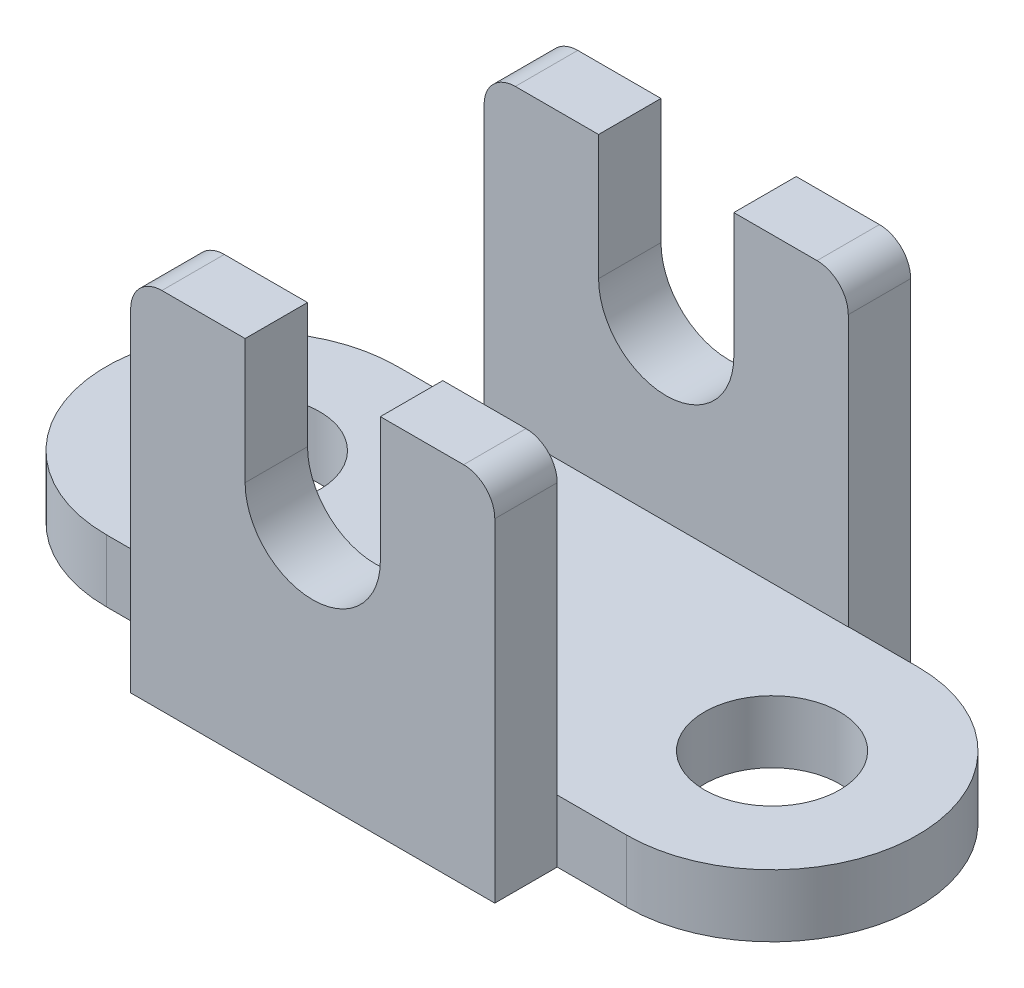
ISO-10303-21;
HEADER;
FILE_DESCRIPTION(('STEP AP214'),'2;1');
FILE_NAME('part.step','',(''),(''),'','','');
FILE_SCHEMA(('AUTOMOTIVE_DESIGN { 1 0 10303 214 1 1 1 1 }'));
ENDSEC;
DATA;
#1=APPLICATION_CONTEXT('core data for automotive mechanical design processes');
#2=APPLICATION_PROTOCOL_DEFINITION('international standard','automotive_design',2000,#1);
#3=PRODUCT_CONTEXT('',#1,'mechanical');
#4=PRODUCT('Part','Part','',(#3));
#5=PRODUCT_RELATED_PRODUCT_CATEGORY('part','',(#4));
#6=PRODUCT_DEFINITION_FORMATION('','',#4);
#7=PRODUCT_DEFINITION_CONTEXT('part definition',#1,'design');
#8=PRODUCT_DEFINITION('design','',#6,#7);
#9=PRODUCT_DEFINITION_SHAPE('','',#8);
#10=(LENGTH_UNIT() NAMED_UNIT(*) SI_UNIT(.MILLI.,.METRE.));
#11=(NAMED_UNIT(*) PLANE_ANGLE_UNIT() SI_UNIT($,.RADIAN.));
#12=(NAMED_UNIT(*) SI_UNIT($,.STERADIAN.) SOLID_ANGLE_UNIT());
#13=UNCERTAINTY_MEASURE_WITH_UNIT(LENGTH_MEASURE(1.E-05),#10,'distance_accuracy_value','');
#14=(GEOMETRIC_REPRESENTATION_CONTEXT(3) GLOBAL_UNCERTAINTY_ASSIGNED_CONTEXT((#13)) GLOBAL_UNIT_ASSIGNED_CONTEXT((#10,
#11,#12)) REPRESENTATION_CONTEXT('',''));
#15=CARTESIAN_POINT('',(0.,0.,0.));
#16=DIRECTION('',(0.,0.,1.));
#17=DIRECTION('',(1.,0.,0.));
#18=AXIS2_PLACEMENT_3D('',#15,#16,#17);
#19=CARTESIAN_POINT('',(-35.5583760815916,6.,33.9743802217869));
#20=DIRECTION('',(0.,0.,1.));
#21=DIRECTION('',(1.,0.,0.));
#22=AXIS2_PLACEMENT_3D('',#19,#20,#21);
#23=PLANE('',#22);
#24=DIRECTION('',(-1.,0.,0.));
#25=VECTOR('',#24,1.);
#26=CARTESIAN_POINT('',(-35.5583760815916,0.,33.9743802217869));
#27=LINE('',#26,#25);
#28=CARTESIAN_POINT('',(-27.2117962466488,0.,33.9743802217869));
#29=VERTEX_POINT('',#28);
#30=CARTESIAN_POINT('',(-35.5583760815916,0.,33.9743802217869));
#31=VERTEX_POINT('',#30);
#32=EDGE_CURVE('E281',#29,#31,#27,.T.);
#33=ORIENTED_EDGE('',*,*,#32,.F.);
#34=DIRECTION('',(0.,1.,0.));
#35=VECTOR('',#34,1.);
#36=CARTESIAN_POINT('',(-27.2117962466488,6.,33.9743802217869));
#37=LINE('',#36,#35);
#38=CARTESIAN_POINT('',(-27.2117962466488,6.,33.9743802217869));
#39=VERTEX_POINT('',#38);
#40=EDGE_CURVE('E11',#29,#39,#37,.T.);
#41=ORIENTED_EDGE('',*,*,#40,.T.);
#42=DIRECTION('',(-1.,0.,0.));
#43=VECTOR('',#42,1.);
#44=CARTESIAN_POINT('',(-35.5583760815916,6.,33.9743802217869));
#45=LINE('',#44,#43);
#46=CARTESIAN_POINT('',(-35.5583760815916,6.,33.9743802217869));
#47=VERTEX_POINT('',#46);
#48=EDGE_CURVE('E271',#39,#47,#45,.T.);
#49=ORIENTED_EDGE('',*,*,#48,.T.);
#50=DIRECTION('',(0.,-1.,0.));
#51=VECTOR('',#50,1.);
#52=CARTESIAN_POINT('',(-35.5583760815916,6.,33.9743802217869));
#53=LINE('',#52,#51);
#54=EDGE_CURVE('E290',#47,#31,#53,.T.);
#55=ORIENTED_EDGE('',*,*,#54,.T.);
#56=EDGE_LOOP('',(#33,#41,#49,#55));
#57=FACE_BOUND('',#56,.T.);
#58=ADVANCED_FACE('F39',(#57),#23,.T.);
#59=CARTESIAN_POINT('',(14.4416239184084,6.,33.9743802217869));
#60=VERTEX_POINT('',#59);
#61=CARTESIAN_POINT('',(7.7882037533512,6.,33.9743802217869));
#62=VERTEX_POINT('',#61);
#63=EDGE_CURVE('E275',#60,#62,#45,.T.);
#64=ORIENTED_EDGE('',*,*,#63,.T.);
#65=DIRECTION('',(0.,1.,0.));
#66=VECTOR('',#65,1.);
#67=CARTESIAN_POINT('',(7.7882037533512,0.,33.9743802217869));
#68=LINE('',#67,#66);
#69=CARTESIAN_POINT('',(7.7882037533512,0.,33.9743802217869));
#70=VERTEX_POINT('',#69);
#71=EDGE_CURVE('E392',#70,#62,#68,.T.);
#72=ORIENTED_EDGE('',*,*,#71,.F.);
#73=CARTESIAN_POINT('',(14.4416239184084,0.,33.9743802217869));
#74=VERTEX_POINT('',#73);
#75=EDGE_CURVE('E262',#74,#70,#27,.T.);
#76=ORIENTED_EDGE('',*,*,#75,.F.);
#77=DIRECTION('',(0.,-1.,0.));
#78=VECTOR('',#77,1.);
#79=CARTESIAN_POINT('',(14.4416239184084,6.,33.9743802217869));
#80=LINE('',#79,#78);
#81=EDGE_CURVE('E292',#60,#74,#80,.T.);
#82=ORIENTED_EDGE('',*,*,#81,.F.);
#83=EDGE_LOOP('',(#64,#72,#76,#82));
#84=FACE_BOUND('',#83,.T.);
#85=ADVANCED_FACE('F388',(#84),#23,.T.);
#86=CARTESIAN_POINT('',(-24.2117962466488,32.,6.));
#87=DIRECTION('',(0.,0.,1.));
#88=DIRECTION('',(1.,0.,0.));
#89=AXIS2_PLACEMENT_3D('',#86,#87,#88);
#90=PLANE('',#89);
#91=DIRECTION('',(0.,-1.,0.));
#92=VECTOR('',#91,1.);
#93=CARTESIAN_POINT('',(-27.2117962466488,0.,6.));
#94=LINE('',#93,#92);
#95=CARTESIAN_POINT('',(-27.2117962466488,32.,6.));
#96=VERTEX_POINT('',#95);
#97=CARTESIAN_POINT('',(-27.2117962466488,6.,6.));
#98=VERTEX_POINT('',#97);
#99=EDGE_CURVE('E301',#96,#98,#94,.T.);
#100=ORIENTED_EDGE('',*,*,#99,.T.);
#101=DIRECTION('',(1.,0.,0.));
#102=VECTOR('',#101,1.);
#103=CARTESIAN_POINT('',(-24.2117962466488,6.,6.));
#104=LINE('',#103,#102);
#105=CARTESIAN_POINT('',(7.7882037533512,6.,6.));
#106=VERTEX_POINT('',#105);
#107=EDGE_CURVE('E371',#98,#106,#104,.T.);
#108=ORIENTED_EDGE('',*,*,#107,.T.);
#109=DIRECTION('',(0.,1.,0.));
#110=VECTOR('',#109,1.);
#111=CARTESIAN_POINT('',(7.7882037533512,0.,6.));
#112=LINE('',#111,#110);
#113=CARTESIAN_POINT('',(7.7882037533512,32.,6.));
#114=VERTEX_POINT('',#113);
#115=EDGE_CURVE('E308',#106,#114,#112,.T.);
#116=ORIENTED_EDGE('',*,*,#115,.T.);
#117=CARTESIAN_POINT('',(4.7882037533512,32.,6.));
#118=DIRECTION('',(0.,0.,1.));
#119=DIRECTION('',(1.,0.,0.));
#120=AXIS2_PLACEMENT_3D('',#117,#118,#119);
#121=CIRCLE('',#120,3.);
#122=CARTESIAN_POINT('',(4.78820375335118,35.,6.));
#123=VERTEX_POINT('',#122);
#124=EDGE_CURVE('E310',#114,#123,#121,.T.);
#125=ORIENTED_EDGE('',*,*,#124,.T.);
#126=DIRECTION('',(-1.,0.,0.));
#127=VECTOR('',#126,1.);
#128=CARTESIAN_POINT('',(-3.2117962466488,35.,6.));
#129=LINE('',#128,#127);
#130=CARTESIAN_POINT('',(-3.2117962466488,35.,6.));
#131=VERTEX_POINT('',#130);
#132=EDGE_CURVE('E313',#123,#131,#129,.T.);
#133=ORIENTED_EDGE('',*,*,#132,.T.);
#134=DIRECTION('',(0.,-1.,0.));
#135=VECTOR('',#134,1.);
#136=CARTESIAN_POINT('',(-3.2117962466488,23.,6.));
#137=LINE('',#136,#135);
#138=CARTESIAN_POINT('',(-3.2117962466488,23.,6.));
#139=VERTEX_POINT('',#138);
#140=EDGE_CURVE('E311',#131,#139,#137,.T.);
#141=ORIENTED_EDGE('',*,*,#140,.T.);
#142=CARTESIAN_POINT('',(-9.7117962466488,23.,6.));
#143=DIRECTION('',(0.,0.,-1.));
#144=DIRECTION('',(1.,0.,0.));
#145=AXIS2_PLACEMENT_3D('',#142,#143,#144);
#146=CIRCLE('',#145,6.5);
#147=CARTESIAN_POINT('',(-16.2117962466488,23.,6.));
#148=VERTEX_POINT('',#147);
#149=EDGE_CURVE('E312',#139,#148,#146,.T.);
#150=ORIENTED_EDGE('',*,*,#149,.T.);
#151=DIRECTION('',(0.,1.,0.));
#152=VECTOR('',#151,1.);
#153=CARTESIAN_POINT('',(-16.2117962466488,35.,6.));
#154=LINE('',#153,#152);
#155=CARTESIAN_POINT('',(-16.2117962466488,35.,6.));
#156=VERTEX_POINT('',#155);
#157=EDGE_CURVE('E320',#148,#156,#154,.T.);
#158=ORIENTED_EDGE('',*,*,#157,.T.);
#159=DIRECTION('',(-1.,0.,0.));
#160=VECTOR('',#159,1.);
#161=CARTESIAN_POINT('',(-24.2117962466488,35.,6.));
#162=LINE('',#161,#160);
#163=CARTESIAN_POINT('',(-24.2117962466488,35.,6.));
#164=VERTEX_POINT('',#163);
#165=EDGE_CURVE('E317',#156,#164,#162,.T.);
#166=ORIENTED_EDGE('',*,*,#165,.T.);
#167=CARTESIAN_POINT('',(-24.2117962466488,32.,6.));
#168=DIRECTION('',(0.,0.,1.));
#169=DIRECTION('',(1.,0.,0.));
#170=AXIS2_PLACEMENT_3D('',#167,#168,#169);
#171=CIRCLE('',#170,3.);
#172=EDGE_CURVE('E321',#164,#96,#171,.T.);
#173=ORIENTED_EDGE('',*,*,#172,.T.);
#174=EDGE_LOOP('',(#100,#108,#116,#125,#133,#141,#150,#158,#166,#173));
#175=FACE_BOUND('',#174,.T.);
#176=ADVANCED_FACE('F533',(#175),#90,.T.);
#177=CARTESIAN_POINT('',(-27.2117962466488,0.,6.));
#178=DIRECTION('',(1.,0.,0.));
#179=DIRECTION('',(0.,0.,-1.));
#180=AXIS2_PLACEMENT_3D('',#177,#178,#179);
#181=PLANE('',#180);
#182=DIRECTION('',(0.,0.,-1.));
#183=VECTOR('',#182,1.);
#184=CARTESIAN_POINT('',(-27.2117962466488,0.,6.));
#185=LINE('',#184,#183);
#186=CARTESIAN_POINT('',(-27.2117962466488,0.,5.97438022178687));
#187=VERTEX_POINT('',#186);
#188=CARTESIAN_POINT('',(-27.2117962466488,0.,0.));
#189=VERTEX_POINT('',#188);
#190=EDGE_CURVE('E369',#187,#189,#185,.T.);
#191=ORIENTED_EDGE('',*,*,#190,.F.);
#192=DIRECTION('',(0.,1.,0.));
#193=VECTOR('',#192,1.);
#194=CARTESIAN_POINT('',(-27.2117962466488,0.,5.97438022178687));
#195=LINE('',#194,#193);
#196=CARTESIAN_POINT('',(-27.2117962466488,6.,5.97438022178687));
#197=VERTEX_POINT('',#196);
#198=EDGE_CURVE('E65',#187,#197,#195,.T.);
#199=ORIENTED_EDGE('',*,*,#198,.T.);
#200=DIRECTION('',(0.,0.,-1.));
#201=VECTOR('',#200,1.);
#202=CARTESIAN_POINT('',(-27.2117962466488,6.,6.));
#203=LINE('',#202,#201);
#204=EDGE_CURVE('E299',#98,#197,#203,.T.);
#205=ORIENTED_EDGE('',*,*,#204,.F.);
#206=ORIENTED_EDGE('',*,*,#99,.F.);
#207=DIRECTION('',(0.,0.,-1.));
#208=VECTOR('',#207,1.);
#209=CARTESIAN_POINT('',(-27.2117962466488,32.,6.));
#210=LINE('',#209,#208);
#211=CARTESIAN_POINT('',(-27.2117962466488,32.,0.));
#212=VERTEX_POINT('',#211);
#213=EDGE_CURVE('E323',#96,#212,#210,.T.);
#214=ORIENTED_EDGE('',*,*,#213,.T.);
#215=DIRECTION('',(0.,-1.,0.));
#216=VECTOR('',#215,1.);
#217=CARTESIAN_POINT('',(-27.2117962466488,0.,0.));
#218=LINE('',#217,#216);
#219=EDGE_CURVE('E305',#212,#189,#218,.T.);
#220=ORIENTED_EDGE('',*,*,#219,.T.);
#221=EDGE_LOOP('',(#191,#199,#205,#206,#214,#220));
#222=FACE_BOUND('',#221,.T.);
#223=ADVANCED_FACE('F41',(#222),#181,.F.);
#224=CARTESIAN_POINT('',(-27.2117962466488,0.,6.));
#225=DIRECTION('',(0.,1.,0.));
#226=DIRECTION('',(0.,0.,1.));
#227=AXIS2_PLACEMENT_3D('',#224,#225,#226);
#228=PLANE('',#227);
#229=CARTESIAN_POINT('',(-35.5583760815916,0.,19.9743802217869));
#230=DIRECTION('',(0.,1.,0.));
#231=DIRECTION('',(0.,0.,1.));
#232=AXIS2_PLACEMENT_3D('',#229,#230,#231);
#233=CIRCLE('',#232,6.5);
#234=CARTESIAN_POINT('',(-35.5583760815916,0.,26.4743802217869));
#235=VERTEX_POINT('',#234);
#236=EDGE_CURVE('E253',#235,#235,#233,.T.);
#237=ORIENTED_EDGE('',*,*,#236,.T.);
#238=EDGE_LOOP('',(#237));
#239=FACE_BOUND('',#238,.T.);
#240=CARTESIAN_POINT('',(14.4416239184084,0.,19.9743802217869));
#241=DIRECTION('',(0.,1.,0.));
#242=DIRECTION('',(0.,0.,1.));
#243=AXIS2_PLACEMENT_3D('',#240,#241,#242);
#244=CIRCLE('',#243,6.5);
#245=CARTESIAN_POINT('',(14.4416239184084,0.,26.4743802217869));
#246=VERTEX_POINT('',#245);
#247=EDGE_CURVE('E245',#246,#246,#244,.T.);
#248=ORIENTED_EDGE('',*,*,#247,.T.);
#249=EDGE_LOOP('',(#248));
#250=FACE_BOUND('',#249,.T.);
#251=DIRECTION('',(1.,0.,0.));
#252=VECTOR('',#251,1.);
#253=CARTESIAN_POINT('',(-35.5583760815916,0.,5.97438022178687));
#254=LINE('',#253,#252);
#255=CARTESIAN_POINT('',(-35.5583760815916,0.,5.97438022178687));
#256=VERTEX_POINT('',#255);
#257=EDGE_CURVE('E278',#256,#187,#254,.T.);
#258=ORIENTED_EDGE('',*,*,#257,.T.);
#259=ORIENTED_EDGE('',*,*,#190,.T.);
#260=DIRECTION('',(1.,0.,0.));
#261=VECTOR('',#260,1.);
#262=CARTESIAN_POINT('',(-27.2117962466488,0.,0.));
#263=LINE('',#262,#261);
#264=CARTESIAN_POINT('',(7.7882037533512,0.,0.));
#265=VERTEX_POINT('',#264);
#266=EDGE_CURVE('E326',#189,#265,#263,.T.);
#267=ORIENTED_EDGE('',*,*,#266,.T.);
#268=DIRECTION('',(0.,0.,-1.));
#269=VECTOR('',#268,1.);
#270=CARTESIAN_POINT('',(7.7882037533512,0.,6.));
#271=LINE('',#270,#269);
#272=CARTESIAN_POINT('',(7.7882037533512,0.,5.97438022178687));
#273=VERTEX_POINT('',#272);
#274=EDGE_CURVE('E370',#273,#265,#271,.T.);
#275=ORIENTED_EDGE('',*,*,#274,.F.);
#276=CARTESIAN_POINT('',(14.4416239184084,0.,5.97438022178687));
#277=VERTEX_POINT('',#276);
#278=EDGE_CURVE('E276',#273,#277,#254,.T.);
#279=ORIENTED_EDGE('',*,*,#278,.T.);
#280=CARTESIAN_POINT('',(14.4416239184084,0.,19.9743802217869));
#281=DIRECTION('',(0.,-1.,0.));
#282=DIRECTION('',(0.,0.,-1.));
#283=AXIS2_PLACEMENT_3D('',#280,#281,#282);
#284=CIRCLE('',#283,14.);
#285=EDGE_CURVE('E285',#277,#74,#284,.T.);
#286=ORIENTED_EDGE('',*,*,#285,.T.);
#287=ORIENTED_EDGE('',*,*,#75,.T.);
#288=DIRECTION('',(0.,0.,-1.));
#289=VECTOR('',#288,1.);
#290=CARTESIAN_POINT('',(7.7882037533512,0.,39.9743802217869));
#291=LINE('',#290,#289);
#292=CARTESIAN_POINT('',(7.7882037533512,0.,39.9743802217869));
#293=VERTEX_POINT('',#292);
#294=EDGE_CURVE('E53',#293,#70,#291,.T.);
#295=ORIENTED_EDGE('',*,*,#294,.F.);
#296=DIRECTION('',(1.,0.,0.));
#297=VECTOR('',#296,1.);
#298=CARTESIAN_POINT('',(-27.2117962466488,0.,39.9743802217869));
#299=LINE('',#298,#297);
#300=CARTESIAN_POINT('',(-27.2117962466488,0.,39.9743802217869));
#301=VERTEX_POINT('',#300);
#302=EDGE_CURVE('E218',#301,#293,#299,.T.);
#303=ORIENTED_EDGE('',*,*,#302,.F.);
#304=DIRECTION('',(0.,0.,-1.));
#305=VECTOR('',#304,1.);
#306=CARTESIAN_POINT('',(-27.2117962466488,0.,39.9743802217869));
#307=LINE('',#306,#305);
#308=EDGE_CURVE('E221',#301,#29,#307,.T.);
#309=ORIENTED_EDGE('',*,*,#308,.T.);
#310=ORIENTED_EDGE('',*,*,#32,.T.);
#311=CARTESIAN_POINT('',(-35.5583760815916,0.,19.9743802217869));
#312=DIRECTION('',(0.,-1.,0.));
#313=DIRECTION('',(0.,0.,-1.));
#314=AXIS2_PLACEMENT_3D('',#311,#312,#313);
#315=CIRCLE('',#314,14.);
#316=EDGE_CURVE('E255',#31,#256,#315,.T.);
#317=ORIENTED_EDGE('',*,*,#316,.T.);
#318=EDGE_LOOP('',(#258,#259,#267,#275,#279,#286,#287,#295,#303,#309,#310,#317));
#319=FACE_BOUND('',#318,.T.);
#320=ADVANCED_FACE('F225',(#239,#250,#319),#228,.F.);
#321=CARTESIAN_POINT('',(7.7882037533512,0.,6.));
#322=DIRECTION('',(-1.,0.,0.));
#323=DIRECTION('',(0.,-1.,0.));
#324=AXIS2_PLACEMENT_3D('',#321,#322,#323);
#325=PLANE('',#324);
#326=DIRECTION('',(0.,0.,1.));
#327=VECTOR('',#326,1.);
#328=CARTESIAN_POINT('',(7.7882037533512,6.,6.));
#329=LINE('',#328,#327);
#330=CARTESIAN_POINT('',(7.7882037533512,6.,5.97438022178687));
#331=VERTEX_POINT('',#330);
#332=EDGE_CURVE('E289',#331,#106,#329,.T.);
#333=ORIENTED_EDGE('',*,*,#332,.F.);
#334=DIRECTION('',(0.,-1.,0.));
#335=VECTOR('',#334,1.);
#336=CARTESIAN_POINT('',(7.7882037533512,0.,5.97438022178687));
#337=LINE('',#336,#335);
#338=EDGE_CURVE('E50',#331,#273,#337,.T.);
#339=ORIENTED_EDGE('',*,*,#338,.T.);
#340=ORIENTED_EDGE('',*,*,#274,.T.);
#341=DIRECTION('',(0.,1.,0.));
#342=VECTOR('',#341,1.);
#343=CARTESIAN_POINT('',(7.7882037533512,0.,0.));
#344=LINE('',#343,#342);
#345=CARTESIAN_POINT('',(7.7882037533512,32.,0.));
#346=VERTEX_POINT('',#345);
#347=EDGE_CURVE('E328',#265,#346,#344,.T.);
#348=ORIENTED_EDGE('',*,*,#347,.T.);
#349=DIRECTION('',(0.,0.,-1.));
#350=VECTOR('',#349,1.);
#351=CARTESIAN_POINT('',(7.7882037533512,32.,6.));
#352=LINE('',#351,#350);
#353=EDGE_CURVE('E365',#114,#346,#352,.T.);
#354=ORIENTED_EDGE('',*,*,#353,.F.);
#355=ORIENTED_EDGE('',*,*,#115,.F.);
#356=EDGE_LOOP('',(#333,#339,#340,#348,#354,#355));
#357=FACE_BOUND('',#356,.T.);
#358=ADVANCED_FACE('F374',(#357),#325,.F.);
#359=CARTESIAN_POINT('',(4.7882037533512,32.,6.));
#360=DIRECTION('',(0.,0.,-1.));
#361=DIRECTION('',(-1.,0.,0.));
#362=AXIS2_PLACEMENT_3D('',#359,#360,#361);
#363=CYLINDRICAL_SURFACE('',#362,3.);
#364=CARTESIAN_POINT('',(4.7882037533512,32.,0.));
#365=DIRECTION('',(0.,0.,1.));
#366=DIRECTION('',(1.,0.,0.));
#367=AXIS2_PLACEMENT_3D('',#364,#365,#366);
#368=CIRCLE('',#367,3.);
#369=CARTESIAN_POINT('',(4.78820375335118,35.,0.));
#370=VERTEX_POINT('',#369);
#371=EDGE_CURVE('E332',#346,#370,#368,.T.);
#372=ORIENTED_EDGE('',*,*,#371,.T.);
#373=DIRECTION('',(0.,0.,-1.));
#374=VECTOR('',#373,1.);
#375=CARTESIAN_POINT('',(4.78820375335118,35.,6.));
#376=LINE('',#375,#374);
#377=EDGE_CURVE('E363',#123,#370,#376,.T.);
#378=ORIENTED_EDGE('',*,*,#377,.F.);
#379=ORIENTED_EDGE('',*,*,#124,.F.);
#380=ORIENTED_EDGE('',*,*,#353,.T.);
#381=EDGE_LOOP('',(#372,#378,#379,#380));
#382=FACE_BOUND('',#381,.T.);
#383=ADVANCED_FACE('F526',(#382),#363,.T.);
#384=CARTESIAN_POINT('',(-3.2117962466488,35.,6.));
#385=DIRECTION('',(0.,-1.,0.));
#386=DIRECTION('',(0.,0.,-1.));
#387=AXIS2_PLACEMENT_3D('',#384,#385,#386);
#388=PLANE('',#387);
#389=DIRECTION('',(-1.,0.,0.));
#390=VECTOR('',#389,1.);
#391=CARTESIAN_POINT('',(-3.2117962466488,35.,0.));
#392=LINE('',#391,#390);
#393=CARTESIAN_POINT('',(-3.2117962466488,35.,0.));
#394=VERTEX_POINT('',#393);
#395=EDGE_CURVE('E334',#370,#394,#392,.T.);
#396=ORIENTED_EDGE('',*,*,#395,.T.);
#397=DIRECTION('',(0.,0.,-1.));
#398=VECTOR('',#397,1.);
#399=CARTESIAN_POINT('',(-3.2117962466488,35.,6.));
#400=LINE('',#399,#398);
#401=EDGE_CURVE('E356',#131,#394,#400,.T.);
#402=ORIENTED_EDGE('',*,*,#401,.F.);
#403=ORIENTED_EDGE('',*,*,#132,.F.);
#404=ORIENTED_EDGE('',*,*,#377,.T.);
#405=EDGE_LOOP('',(#396,#402,#403,#404));
#406=FACE_BOUND('',#405,.T.);
#407=ADVANCED_FACE('F522',(#406),#388,.F.);
#408=CARTESIAN_POINT('',(-3.2117962466488,23.,6.));
#409=DIRECTION('',(1.,0.,0.));
#410=DIRECTION('',(0.,1.,0.));
#411=AXIS2_PLACEMENT_3D('',#408,#409,#410);
#412=PLANE('',#411);
#413=DIRECTION('',(0.,-1.,0.));
#414=VECTOR('',#413,1.);
#415=CARTESIAN_POINT('',(-3.2117962466488,23.,0.));
#416=LINE('',#415,#414);
#417=CARTESIAN_POINT('',(-3.2117962466488,23.,0.));
#418=VERTEX_POINT('',#417);
#419=EDGE_CURVE('E333',#394,#418,#416,.T.);
#420=ORIENTED_EDGE('',*,*,#419,.T.);
#421=DIRECTION('',(0.,0.,-1.));
#422=VECTOR('',#421,1.);
#423=CARTESIAN_POINT('',(-3.2117962466488,23.,6.));
#424=LINE('',#423,#422);
#425=EDGE_CURVE('E351',#139,#418,#424,.T.);
#426=ORIENTED_EDGE('',*,*,#425,.F.);
#427=ORIENTED_EDGE('',*,*,#140,.F.);
#428=ORIENTED_EDGE('',*,*,#401,.T.);
#429=EDGE_LOOP('',(#420,#426,#427,#428));
#430=FACE_BOUND('',#429,.T.);
#431=ADVANCED_FACE('F519',(#430),#412,.F.);
#432=CARTESIAN_POINT('',(-9.7117962466488,23.,6.));
#433=DIRECTION('',(0.,0.,-1.));
#434=DIRECTION('',(-1.,0.,0.));
#435=AXIS2_PLACEMENT_3D('',#432,#433,#434);
#436=CYLINDRICAL_SURFACE('',#435,6.5);
#437=CARTESIAN_POINT('',(-9.7117962466488,23.,0.));
#438=DIRECTION('',(0.,0.,-1.));
#439=DIRECTION('',(1.,0.,0.));
#440=AXIS2_PLACEMENT_3D('',#437,#438,#439);
#441=CIRCLE('',#440,6.5);
#442=CARTESIAN_POINT('',(-16.2117962466488,23.,0.));
#443=VERTEX_POINT('',#442);
#444=EDGE_CURVE('E340',#418,#443,#441,.T.);
#445=ORIENTED_EDGE('',*,*,#444,.T.);
#446=DIRECTION('',(0.,0.,-1.));
#447=VECTOR('',#446,1.);
#448=CARTESIAN_POINT('',(-16.2117962466488,23.,6.));
#449=LINE('',#448,#447);
#450=EDGE_CURVE('E355',#148,#443,#449,.T.);
#451=ORIENTED_EDGE('',*,*,#450,.F.);
#452=ORIENTED_EDGE('',*,*,#149,.F.);
#453=ORIENTED_EDGE('',*,*,#425,.T.);
#454=EDGE_LOOP('',(#445,#451,#452,#453));
#455=FACE_BOUND('',#454,.T.);
#456=ADVANCED_FACE('F514',(#455),#436,.F.);
#457=CARTESIAN_POINT('',(-16.2117962466488,35.,6.));
#458=DIRECTION('',(-1.,0.,0.));
#459=DIRECTION('',(0.,-1.,0.));
#460=AXIS2_PLACEMENT_3D('',#457,#458,#459);
#461=PLANE('',#460);
#462=DIRECTION('',(0.,1.,0.));
#463=VECTOR('',#462,1.);
#464=CARTESIAN_POINT('',(-16.2117962466488,35.,0.));
#465=LINE('',#464,#463);
#466=CARTESIAN_POINT('',(-16.2117962466488,35.,0.));
#467=VERTEX_POINT('',#466);
#468=EDGE_CURVE('E339',#443,#467,#465,.T.);
#469=ORIENTED_EDGE('',*,*,#468,.T.);
#470=DIRECTION('',(0.,0.,-1.));
#471=VECTOR('',#470,1.);
#472=CARTESIAN_POINT('',(-16.2117962466488,35.,6.));
#473=LINE('',#472,#471);
#474=EDGE_CURVE('E349',#156,#467,#473,.T.);
#475=ORIENTED_EDGE('',*,*,#474,.F.);
#476=ORIENTED_EDGE('',*,*,#157,.F.);
#477=ORIENTED_EDGE('',*,*,#450,.T.);
#478=EDGE_LOOP('',(#469,#475,#476,#477));
#479=FACE_BOUND('',#478,.T.);
#480=ADVANCED_FACE('F509',(#479),#461,.F.);
#481=CARTESIAN_POINT('',(-24.2117962466488,35.,6.));
#482=DIRECTION('',(0.,-1.,0.));
#483=DIRECTION('',(0.,0.,-1.));
#484=AXIS2_PLACEMENT_3D('',#481,#482,#483);
#485=PLANE('',#484);
#486=DIRECTION('',(-1.,0.,0.));
#487=VECTOR('',#486,1.);
#488=CARTESIAN_POINT('',(-24.2117962466488,35.,0.));
#489=LINE('',#488,#487);
#490=CARTESIAN_POINT('',(-24.2117962466488,35.,0.));
#491=VERTEX_POINT('',#490);
#492=EDGE_CURVE('E343',#467,#491,#489,.T.);
#493=ORIENTED_EDGE('',*,*,#492,.T.);
#494=DIRECTION('',(0.,0.,-1.));
#495=VECTOR('',#494,1.);
#496=CARTESIAN_POINT('',(-24.2117962466488,35.,6.));
#497=LINE('',#496,#495);
#498=EDGE_CURVE('E347',#164,#491,#497,.T.);
#499=ORIENTED_EDGE('',*,*,#498,.F.);
#500=ORIENTED_EDGE('',*,*,#165,.F.);
#501=ORIENTED_EDGE('',*,*,#474,.T.);
#502=EDGE_LOOP('',(#493,#499,#500,#501));
#503=FACE_BOUND('',#502,.T.);
#504=ADVANCED_FACE('F501',(#503),#485,.F.);
#505=CARTESIAN_POINT('',(-24.2117962466488,32.,6.));
#506=DIRECTION('',(0.,0.,-1.));
#507=DIRECTION('',(-1.,0.,0.));
#508=AXIS2_PLACEMENT_3D('',#505,#506,#507);
#509=CYLINDRICAL_SURFACE('',#508,3.);
#510=CARTESIAN_POINT('',(-24.2117962466488,32.,0.));
#511=DIRECTION('',(0.,0.,1.));
#512=DIRECTION('',(1.,0.,0.));
#513=AXIS2_PLACEMENT_3D('',#510,#511,#512);
#514=CIRCLE('',#513,3.);
#515=EDGE_CURVE('E307',#491,#212,#514,.T.);
#516=ORIENTED_EDGE('',*,*,#515,.T.);
#517=ORIENTED_EDGE('',*,*,#213,.F.);
#518=ORIENTED_EDGE('',*,*,#172,.F.);
#519=ORIENTED_EDGE('',*,*,#498,.T.);
#520=EDGE_LOOP('',(#516,#517,#518,#519));
#521=FACE_BOUND('',#520,.T.);
#522=ADVANCED_FACE('F496',(#521),#509,.T.);
#523=CARTESIAN_POINT('',(-24.2117962466488,32.,0.));
#524=DIRECTION('',(0.,0.,1.));
#525=DIRECTION('',(1.,0.,0.));
#526=AXIS2_PLACEMENT_3D('',#523,#524,#525);
#527=PLANE('',#526);
#528=ORIENTED_EDGE('',*,*,#219,.F.);
#529=ORIENTED_EDGE('',*,*,#515,.F.);
#530=ORIENTED_EDGE('',*,*,#492,.F.);
#531=ORIENTED_EDGE('',*,*,#468,.F.);
#532=ORIENTED_EDGE('',*,*,#444,.F.);
#533=ORIENTED_EDGE('',*,*,#419,.F.);
#534=ORIENTED_EDGE('',*,*,#395,.F.);
#535=ORIENTED_EDGE('',*,*,#371,.F.);
#536=ORIENTED_EDGE('',*,*,#347,.F.);
#537=ORIENTED_EDGE('',*,*,#266,.F.);
#538=EDGE_LOOP('',(#528,#529,#530,#531,#532,#533,#534,#535,#536,#537));
#539=FACE_BOUND('',#538,.T.);
#540=ADVANCED_FACE('F495',(#539),#527,.F.);
#541=CARTESIAN_POINT('',(-35.5583760815916,6.,5.97438022178687));
#542=DIRECTION('',(0.,0.,-1.));
#543=DIRECTION('',(-1.,0.,0.));
#544=AXIS2_PLACEMENT_3D('',#541,#542,#543);
#545=PLANE('',#544);
#546=ORIENTED_EDGE('',*,*,#198,.F.);
#547=ORIENTED_EDGE('',*,*,#257,.F.);
#548=DIRECTION('',(0.,-1.,0.));
#549=VECTOR('',#548,1.);
#550=CARTESIAN_POINT('',(-35.5583760815916,6.,5.97438022178687));
#551=LINE('',#550,#549);
#552=CARTESIAN_POINT('',(-35.5583760815916,6.,5.97438022178687));
#553=VERTEX_POINT('',#552);
#554=EDGE_CURVE('E274',#553,#256,#551,.T.);
#555=ORIENTED_EDGE('',*,*,#554,.F.);
#556=DIRECTION('',(1.,0.,0.));
#557=VECTOR('',#556,1.);
#558=CARTESIAN_POINT('',(-35.5583760815916,6.,5.97438022178687));
#559=LINE('',#558,#557);
#560=EDGE_CURVE('E264',#553,#197,#559,.T.);
#561=ORIENTED_EDGE('',*,*,#560,.T.);
#562=EDGE_LOOP('',(#546,#547,#555,#561));
#563=FACE_BOUND('',#562,.T.);
#564=ADVANCED_FACE('F488',(#563),#545,.T.);
#565=ORIENTED_EDGE('',*,*,#338,.F.);
#566=CARTESIAN_POINT('',(14.4416239184084,6.,5.97438022178687));
#567=VERTEX_POINT('',#566);
#568=EDGE_CURVE('E263',#331,#567,#559,.T.);
#569=ORIENTED_EDGE('',*,*,#568,.T.);
#570=DIRECTION('',(0.,-1.,0.));
#571=VECTOR('',#570,1.);
#572=CARTESIAN_POINT('',(14.4416239184084,6.,5.97438022178687));
#573=LINE('',#572,#571);
#574=EDGE_CURVE('E291',#567,#277,#573,.T.);
#575=ORIENTED_EDGE('',*,*,#574,.T.);
#576=ORIENTED_EDGE('',*,*,#278,.F.);
#577=EDGE_LOOP('',(#565,#569,#575,#576));
#578=FACE_BOUND('',#577,.T.);
#579=ADVANCED_FACE('F385',(#578),#545,.T.);
#580=CARTESIAN_POINT('',(-35.5583760815916,6.,19.9743802217869));
#581=DIRECTION('',(0.,-1.,0.));
#582=DIRECTION('',(0.,0.,-1.));
#583=AXIS2_PLACEMENT_3D('',#580,#581,#582);
#584=PLANE('',#583);
#585=CARTESIAN_POINT('',(-35.5583760815916,6.,19.9743802217869));
#586=DIRECTION('',(0.,1.,0.));
#587=DIRECTION('',(0.,0.,1.));
#588=AXIS2_PLACEMENT_3D('',#585,#586,#587);
#589=CIRCLE('',#588,6.5);
#590=CARTESIAN_POINT('',(-35.5583760815916,6.,26.4743802217869));
#591=VERTEX_POINT('',#590);
#592=EDGE_CURVE('E254',#591,#591,#589,.T.);
#593=ORIENTED_EDGE('',*,*,#592,.F.);
#594=EDGE_LOOP('',(#593));
#595=FACE_BOUND('',#594,.T.);
#596=CARTESIAN_POINT('',(14.4416239184084,6.,19.9743802217869));
#597=DIRECTION('',(0.,1.,0.));
#598=DIRECTION('',(0.,0.,1.));
#599=AXIS2_PLACEMENT_3D('',#596,#597,#598);
#600=CIRCLE('',#599,6.5);
#601=CARTESIAN_POINT('',(14.4416239184084,6.,26.4743802217869));
#602=VERTEX_POINT('',#601);
#603=EDGE_CURVE('E241',#602,#602,#600,.T.);
#604=ORIENTED_EDGE('',*,*,#603,.F.);
#605=EDGE_LOOP('',(#604));
#606=FACE_BOUND('',#605,.T.);
#607=ORIENTED_EDGE('',*,*,#107,.F.);
#608=ORIENTED_EDGE('',*,*,#204,.T.);
#609=ORIENTED_EDGE('',*,*,#560,.F.);
#610=CARTESIAN_POINT('',(-35.5583760815916,6.,19.9743802217869));
#611=DIRECTION('',(0.,-1.,0.));
#612=DIRECTION('',(0.,0.,-1.));
#613=AXIS2_PLACEMENT_3D('',#610,#611,#612);
#614=CIRCLE('',#613,14.);
#615=EDGE_CURVE('E257',#47,#553,#614,.T.);
#616=ORIENTED_EDGE('',*,*,#615,.F.);
#617=ORIENTED_EDGE('',*,*,#48,.F.);
#618=EDGE_CURVE('E277',#62,#39,#45,.T.);
#619=ORIENTED_EDGE('',*,*,#618,.F.);
#620=ORIENTED_EDGE('',*,*,#63,.F.);
#621=CARTESIAN_POINT('',(14.4416239184084,6.,19.9743802217869));
#622=DIRECTION('',(0.,-1.,0.));
#623=DIRECTION('',(0.,0.,-1.));
#624=AXIS2_PLACEMENT_3D('',#621,#622,#623);
#625=CIRCLE('',#624,14.);
#626=EDGE_CURVE('E268',#567,#60,#625,.T.);
#627=ORIENTED_EDGE('',*,*,#626,.F.);
#628=ORIENTED_EDGE('',*,*,#568,.F.);
#629=ORIENTED_EDGE('',*,*,#332,.T.);
#630=EDGE_LOOP('',(#607,#608,#609,#616,#617,#619,#620,#627,#628,#629));
#631=FACE_BOUND('',#630,.T.);
#632=ADVANCED_FACE('F486',(#595,#606,#631),#584,.F.);
#633=CARTESIAN_POINT('',(-35.5583760815916,6.,19.9743802217869));
#634=DIRECTION('',(0.,-1.,0.));
#635=DIRECTION('',(0.,0.,-1.));
#636=AXIS2_PLACEMENT_3D('',#633,#634,#635);
#637=CYLINDRICAL_SURFACE('',#636,14.);
#638=ORIENTED_EDGE('',*,*,#316,.F.);
#639=ORIENTED_EDGE('',*,*,#54,.F.);
#640=ORIENTED_EDGE('',*,*,#615,.T.);
#641=ORIENTED_EDGE('',*,*,#554,.T.);
#642=EDGE_LOOP('',(#638,#639,#640,#641));
#643=FACE_BOUND('',#642,.T.);
#644=ADVANCED_FACE('F483',(#643),#637,.T.);
#645=CARTESIAN_POINT('',(14.4416239184084,6.,19.9743802217869));
#646=DIRECTION('',(0.,-1.,0.));
#647=DIRECTION('',(0.,0.,-1.));
#648=AXIS2_PLACEMENT_3D('',#645,#646,#647);
#649=CYLINDRICAL_SURFACE('',#648,14.);
#650=ORIENTED_EDGE('',*,*,#285,.F.);
#651=ORIENTED_EDGE('',*,*,#574,.F.);
#652=ORIENTED_EDGE('',*,*,#626,.T.);
#653=ORIENTED_EDGE('',*,*,#81,.T.);
#654=EDGE_LOOP('',(#650,#651,#652,#653));
#655=FACE_BOUND('',#654,.T.);
#656=ADVANCED_FACE('F390',(#655),#649,.T.);
#657=CARTESIAN_POINT('',(14.4416239184084,0.,19.9743802217869));
#658=DIRECTION('',(0.,1.,0.));
#659=DIRECTION('',(0.,0.,1.));
#660=AXIS2_PLACEMENT_3D('',#657,#658,#659);
#661=CYLINDRICAL_SURFACE('',#660,6.5);
#662=ORIENTED_EDGE('',*,*,#247,.F.);
#663=EDGE_LOOP('',(#662));
#664=FACE_BOUND('',#663,.T.);
#665=ORIENTED_EDGE('',*,*,#603,.T.);
#666=EDGE_LOOP('',(#665));
#667=FACE_BOUND('',#666,.T.);
#668=ADVANCED_FACE('F552',(#664,#667),#661,.F.);
#669=CARTESIAN_POINT('',(-35.5583760815916,0.,19.9743802217869));
#670=DIRECTION('',(0.,1.,0.));
#671=DIRECTION('',(0.,0.,1.));
#672=AXIS2_PLACEMENT_3D('',#669,#670,#671);
#673=CYLINDRICAL_SURFACE('',#672,6.5);
#674=ORIENTED_EDGE('',*,*,#236,.F.);
#675=EDGE_LOOP('',(#674));
#676=FACE_BOUND('',#675,.T.);
#677=ORIENTED_EDGE('',*,*,#592,.T.);
#678=EDGE_LOOP('',(#677));
#679=FACE_BOUND('',#678,.T.);
#680=ADVANCED_FACE('F566',(#676,#679),#673,.F.);
#681=CARTESIAN_POINT('',(4.7882037533512,32.,33.9743802217869));
#682=DIRECTION('',(0.,0.,1.));
#683=DIRECTION('',(1.,0.,0.));
#684=AXIS2_PLACEMENT_3D('',#681,#682,#683);
#685=PLANE('',#684);
#686=CARTESIAN_POINT('',(7.7882037533512,32.,33.9743802217869));
#687=VERTEX_POINT('',#686);
#688=EDGE_CURVE('E391',#62,#687,#68,.T.);
#689=ORIENTED_EDGE('',*,*,#688,.F.);
#690=ORIENTED_EDGE('',*,*,#618,.T.);
#691=DIRECTION('',(0.,-1.,0.));
#692=VECTOR('',#691,1.);
#693=CARTESIAN_POINT('',(-27.2117962466488,32.,33.9743802217869));
#694=LINE('',#693,#692);
#695=CARTESIAN_POINT('',(-27.2117962466488,32.,33.9743802217869));
#696=VERTEX_POINT('',#695);
#697=EDGE_CURVE('E397',#696,#39,#694,.T.);
#698=ORIENTED_EDGE('',*,*,#697,.F.);
#699=CARTESIAN_POINT('',(-24.2117962466488,32.,33.9743802217869));
#700=DIRECTION('',(0.,0.,1.));
#701=DIRECTION('',(1.,0.,0.));
#702=AXIS2_PLACEMENT_3D('',#699,#700,#701);
#703=CIRCLE('',#702,3.);
#704=CARTESIAN_POINT('',(-24.2117962466488,35.,33.9743802217869));
#705=VERTEX_POINT('',#704);
#706=EDGE_CURVE('E236',#705,#696,#703,.T.);
#707=ORIENTED_EDGE('',*,*,#706,.F.);
#708=DIRECTION('',(-1.,0.,0.));
#709=VECTOR('',#708,1.);
#710=CARTESIAN_POINT('',(-16.2117962466488,35.,33.9743802217869));
#711=LINE('',#710,#709);
#712=CARTESIAN_POINT('',(-16.2117962466488,35.,33.9743802217869));
#713=VERTEX_POINT('',#712);
#714=EDGE_CURVE('E406',#713,#705,#711,.T.);
#715=ORIENTED_EDGE('',*,*,#714,.F.);
#716=DIRECTION('',(0.,1.,0.));
#717=VECTOR('',#716,1.);
#718=CARTESIAN_POINT('',(-16.2117962466488,35.,33.9743802217869));
#719=LINE('',#718,#717);
#720=CARTESIAN_POINT('',(-16.2117962466488,23.,33.9743802217869));
#721=VERTEX_POINT('',#720);
#722=EDGE_CURVE('E408',#721,#713,#719,.T.);
#723=ORIENTED_EDGE('',*,*,#722,.F.);
#724=CARTESIAN_POINT('',(-9.7117962466488,23.,33.9743802217869));
#725=DIRECTION('',(0.,0.,-1.));
#726=DIRECTION('',(1.,0.,0.));
#727=AXIS2_PLACEMENT_3D('',#724,#725,#726);
#728=CIRCLE('',#727,6.5);
#729=CARTESIAN_POINT('',(-3.2117962466488,23.,33.9743802217869));
#730=VERTEX_POINT('',#729);
#731=EDGE_CURVE('E407',#730,#721,#728,.T.);
#732=ORIENTED_EDGE('',*,*,#731,.F.);
#733=DIRECTION('',(0.,-1.,0.));
#734=VECTOR('',#733,1.);
#735=CARTESIAN_POINT('',(-3.2117962466488,23.,33.9743802217869));
#736=LINE('',#735,#734);
#737=CARTESIAN_POINT('',(-3.2117962466488,35.,33.9743802217869));
#738=VERTEX_POINT('',#737);
#739=EDGE_CURVE('E404',#738,#730,#736,.T.);
#740=ORIENTED_EDGE('',*,*,#739,.F.);
#741=DIRECTION('',(-1.,0.,0.));
#742=VECTOR('',#741,1.);
#743=CARTESIAN_POINT('',(4.78820375335118,35.,33.9743802217869));
#744=LINE('',#743,#742);
#745=CARTESIAN_POINT('',(4.78820375335118,35.,33.9743802217869));
#746=VERTEX_POINT('',#745);
#747=EDGE_CURVE('E400',#746,#738,#744,.T.);
#748=ORIENTED_EDGE('',*,*,#747,.F.);
#749=CARTESIAN_POINT('',(4.7882037533512,32.,33.9743802217869));
#750=DIRECTION('',(0.,0.,1.));
#751=DIRECTION('',(1.,0.,0.));
#752=AXIS2_PLACEMENT_3D('',#749,#750,#751);
#753=CIRCLE('',#752,3.);
#754=EDGE_CURVE('E394',#687,#746,#753,.T.);
#755=ORIENTED_EDGE('',*,*,#754,.F.);
#756=EDGE_LOOP('',(#689,#690,#698,#707,#715,#723,#732,#740,#748,#755));
#757=FACE_BOUND('',#756,.T.);
#758=ADVANCED_FACE('F445',(#757),#685,.F.);
#759=CARTESIAN_POINT('',(-27.2117962466488,32.,39.9743802217869));
#760=DIRECTION('',(1.,0.,0.));
#761=DIRECTION('',(0.,0.,-1.));
#762=AXIS2_PLACEMENT_3D('',#759,#760,#761);
#763=PLANE('',#762);
#764=ORIENTED_EDGE('',*,*,#697,.T.);
#765=ORIENTED_EDGE('',*,*,#40,.F.);
#766=ORIENTED_EDGE('',*,*,#308,.F.);
#767=DIRECTION('',(0.,-1.,0.));
#768=VECTOR('',#767,1.);
#769=CARTESIAN_POINT('',(-27.2117962466488,32.,39.9743802217869));
#770=LINE('',#769,#768);
#771=CARTESIAN_POINT('',(-27.2117962466488,32.,39.9743802217869));
#772=VERTEX_POINT('',#771);
#773=EDGE_CURVE('E229',#772,#301,#770,.T.);
#774=ORIENTED_EDGE('',*,*,#773,.F.);
#775=DIRECTION('',(0.,0.,-1.));
#776=VECTOR('',#775,1.);
#777=CARTESIAN_POINT('',(-27.2117962466488,32.,39.9743802217869));
#778=LINE('',#777,#776);
#779=EDGE_CURVE('E411',#772,#696,#778,.T.);
#780=ORIENTED_EDGE('',*,*,#779,.T.);
#781=EDGE_LOOP('',(#764,#765,#766,#774,#780));
#782=FACE_BOUND('',#781,.T.);
#783=ADVANCED_FACE('F242',(#782),#763,.F.);
#784=CARTESIAN_POINT('',(7.7882037533512,0.,39.9743802217869));
#785=DIRECTION('',(-1.,0.,0.));
#786=DIRECTION('',(0.,0.,1.));
#787=AXIS2_PLACEMENT_3D('',#784,#785,#786);
#788=PLANE('',#787);
#789=ORIENTED_EDGE('',*,*,#71,.T.);
#790=ORIENTED_EDGE('',*,*,#688,.T.);
#791=DIRECTION('',(0.,0.,-1.));
#792=VECTOR('',#791,1.);
#793=CARTESIAN_POINT('',(7.7882037533512,32.,39.9743802217869));
#794=LINE('',#793,#792);
#795=CARTESIAN_POINT('',(7.7882037533512,32.,39.9743802217869));
#796=VERTEX_POINT('',#795);
#797=EDGE_CURVE('E250',#796,#687,#794,.T.);
#798=ORIENTED_EDGE('',*,*,#797,.F.);
#799=DIRECTION('',(0.,1.,0.));
#800=VECTOR('',#799,1.);
#801=CARTESIAN_POINT('',(7.7882037533512,0.,39.9743802217869));
#802=LINE('',#801,#800);
#803=EDGE_CURVE('E228',#293,#796,#802,.T.);
#804=ORIENTED_EDGE('',*,*,#803,.F.);
#805=ORIENTED_EDGE('',*,*,#294,.T.);
#806=EDGE_LOOP('',(#789,#790,#798,#804,#805));
#807=FACE_BOUND('',#806,.T.);
#808=ADVANCED_FACE('F576',(#807),#788,.F.);
#809=CARTESIAN_POINT('',(4.7882037533512,32.,39.9743802217869));
#810=DIRECTION('',(0.,0.,-1.));
#811=DIRECTION('',(-1.,0.,0.));
#812=AXIS2_PLACEMENT_3D('',#809,#810,#811);
#813=CYLINDRICAL_SURFACE('',#812,3.);
#814=ORIENTED_EDGE('',*,*,#754,.T.);
#815=DIRECTION('',(0.,0.,-1.));
#816=VECTOR('',#815,1.);
#817=CARTESIAN_POINT('',(4.78820375335118,35.,39.9743802217869));
#818=LINE('',#817,#816);
#819=CARTESIAN_POINT('',(4.78820375335118,35.,39.9743802217869));
#820=VERTEX_POINT('',#819);
#821=EDGE_CURVE('E429',#820,#746,#818,.T.);
#822=ORIENTED_EDGE('',*,*,#821,.F.);
#823=CARTESIAN_POINT('',(4.7882037533512,32.,39.9743802217869));
#824=DIRECTION('',(0.,0.,1.));
#825=DIRECTION('',(1.,0.,0.));
#826=AXIS2_PLACEMENT_3D('',#823,#824,#825);
#827=CIRCLE('',#826,3.);
#828=EDGE_CURVE('E438',#796,#820,#827,.T.);
#829=ORIENTED_EDGE('',*,*,#828,.F.);
#830=ORIENTED_EDGE('',*,*,#797,.T.);
#831=EDGE_LOOP('',(#814,#822,#829,#830));
#832=FACE_BOUND('',#831,.T.);
#833=ADVANCED_FACE('F440',(#832),#813,.T.);
#834=CARTESIAN_POINT('',(4.78820375335118,35.,39.9743802217869));
#835=DIRECTION('',(0.,-1.,0.));
#836=DIRECTION('',(0.,0.,-1.));
#837=AXIS2_PLACEMENT_3D('',#834,#835,#836);
#838=PLANE('',#837);
#839=ORIENTED_EDGE('',*,*,#747,.T.);
#840=DIRECTION('',(0.,0.,-1.));
#841=VECTOR('',#840,1.);
#842=CARTESIAN_POINT('',(-3.2117962466488,35.,39.9743802217869));
#843=LINE('',#842,#841);
#844=CARTESIAN_POINT('',(-3.2117962466488,35.,39.9743802217869));
#845=VERTEX_POINT('',#844);
#846=EDGE_CURVE('E430',#845,#738,#843,.T.);
#847=ORIENTED_EDGE('',*,*,#846,.F.);
#848=DIRECTION('',(-1.,0.,0.));
#849=VECTOR('',#848,1.);
#850=CARTESIAN_POINT('',(4.78820375335118,35.,39.9743802217869));
#851=LINE('',#850,#849);
#852=EDGE_CURVE('E457',#820,#845,#851,.T.);
#853=ORIENTED_EDGE('',*,*,#852,.F.);
#854=ORIENTED_EDGE('',*,*,#821,.T.);
#855=EDGE_LOOP('',(#839,#847,#853,#854));
#856=FACE_BOUND('',#855,.T.);
#857=ADVANCED_FACE('F450',(#856),#838,.F.);
#858=CARTESIAN_POINT('',(-3.2117962466488,23.,39.9743802217869));
#859=DIRECTION('',(1.,0.,0.));
#860=DIRECTION('',(0.,1.,0.));
#861=AXIS2_PLACEMENT_3D('',#858,#859,#860);
#862=PLANE('',#861);
#863=ORIENTED_EDGE('',*,*,#739,.T.);
#864=DIRECTION('',(0.,0.,-1.));
#865=VECTOR('',#864,1.);
#866=CARTESIAN_POINT('',(-3.2117962466488,23.,39.9743802217869));
#867=LINE('',#866,#865);
#868=CARTESIAN_POINT('',(-3.2117962466488,23.,39.9743802217869));
#869=VERTEX_POINT('',#868);
#870=EDGE_CURVE('E424',#869,#730,#867,.T.);
#871=ORIENTED_EDGE('',*,*,#870,.F.);
#872=DIRECTION('',(0.,-1.,0.));
#873=VECTOR('',#872,1.);
#874=CARTESIAN_POINT('',(-3.2117962466488,23.,39.9743802217869));
#875=LINE('',#874,#873);
#876=EDGE_CURVE('E451',#845,#869,#875,.T.);
#877=ORIENTED_EDGE('',*,*,#876,.F.);
#878=ORIENTED_EDGE('',*,*,#846,.T.);
#879=EDGE_LOOP('',(#863,#871,#877,#878));
#880=FACE_BOUND('',#879,.T.);
#881=ADVANCED_FACE('F453',(#880),#862,.F.);
#882=CARTESIAN_POINT('',(-9.7117962466488,23.,39.9743802217869));
#883=DIRECTION('',(0.,0.,-1.));
#884=DIRECTION('',(-1.,0.,0.));
#885=AXIS2_PLACEMENT_3D('',#882,#883,#884);
#886=CYLINDRICAL_SURFACE('',#885,6.5);
#887=ORIENTED_EDGE('',*,*,#731,.T.);
#888=DIRECTION('',(0.,0.,-1.));
#889=VECTOR('',#888,1.);
#890=CARTESIAN_POINT('',(-16.2117962466488,23.,39.9743802217869));
#891=LINE('',#890,#889);
#892=CARTESIAN_POINT('',(-16.2117962466488,23.,39.9743802217869));
#893=VERTEX_POINT('',#892);
#894=EDGE_CURVE('E423',#893,#721,#891,.T.);
#895=ORIENTED_EDGE('',*,*,#894,.F.);
#896=CARTESIAN_POINT('',(-9.7117962466488,23.,39.9743802217869));
#897=DIRECTION('',(0.,0.,-1.));
#898=DIRECTION('',(1.,0.,0.));
#899=AXIS2_PLACEMENT_3D('',#896,#897,#898);
#900=CIRCLE('',#899,6.5);
#901=EDGE_CURVE('E454',#869,#893,#900,.T.);
#902=ORIENTED_EDGE('',*,*,#901,.F.);
#903=ORIENTED_EDGE('',*,*,#870,.T.);
#904=EDGE_LOOP('',(#887,#895,#902,#903));
#905=FACE_BOUND('',#904,.T.);
#906=ADVANCED_FACE('F590',(#905),#886,.F.);
#907=CARTESIAN_POINT('',(-16.2117962466488,35.,39.9743802217869));
#908=DIRECTION('',(-1.,0.,0.));
#909=DIRECTION('',(0.,-1.,0.));
#910=AXIS2_PLACEMENT_3D('',#907,#908,#909);
#911=PLANE('',#910);
#912=ORIENTED_EDGE('',*,*,#722,.T.);
#913=DIRECTION('',(0.,0.,-1.));
#914=VECTOR('',#913,1.);
#915=CARTESIAN_POINT('',(-16.2117962466488,35.,39.9743802217869));
#916=LINE('',#915,#914);
#917=CARTESIAN_POINT('',(-16.2117962466488,35.,39.9743802217869));
#918=VERTEX_POINT('',#917);
#919=EDGE_CURVE('E416',#918,#713,#916,.T.);
#920=ORIENTED_EDGE('',*,*,#919,.F.);
#921=DIRECTION('',(0.,1.,0.));
#922=VECTOR('',#921,1.);
#923=CARTESIAN_POINT('',(-16.2117962466488,35.,39.9743802217869));
#924=LINE('',#923,#922);
#925=EDGE_CURVE('E456',#893,#918,#924,.T.);
#926=ORIENTED_EDGE('',*,*,#925,.F.);
#927=ORIENTED_EDGE('',*,*,#894,.T.);
#928=EDGE_LOOP('',(#912,#920,#926,#927));
#929=FACE_BOUND('',#928,.T.);
#930=ADVANCED_FACE('F587',(#929),#911,.F.);
#931=CARTESIAN_POINT('',(-16.2117962466488,35.,39.9743802217869));
#932=DIRECTION('',(0.,-1.,0.));
#933=DIRECTION('',(0.,0.,-1.));
#934=AXIS2_PLACEMENT_3D('',#931,#932,#933);
#935=PLANE('',#934);
#936=ORIENTED_EDGE('',*,*,#714,.T.);
#937=DIRECTION('',(0.,0.,-1.));
#938=VECTOR('',#937,1.);
#939=CARTESIAN_POINT('',(-24.2117962466488,35.,39.9743802217869));
#940=LINE('',#939,#938);
#941=CARTESIAN_POINT('',(-24.2117962466488,35.,39.9743802217869));
#942=VERTEX_POINT('',#941);
#943=EDGE_CURVE('E414',#942,#705,#940,.T.);
#944=ORIENTED_EDGE('',*,*,#943,.F.);
#945=DIRECTION('',(-1.,0.,0.));
#946=VECTOR('',#945,1.);
#947=CARTESIAN_POINT('',(-16.2117962466488,35.,39.9743802217869));
#948=LINE('',#947,#946);
#949=EDGE_CURVE('E464',#918,#942,#948,.T.);
#950=ORIENTED_EDGE('',*,*,#949,.F.);
#951=ORIENTED_EDGE('',*,*,#919,.T.);
#952=EDGE_LOOP('',(#936,#944,#950,#951));
#953=FACE_BOUND('',#952,.T.);
#954=ADVANCED_FACE('F469',(#953),#935,.F.);
#955=CARTESIAN_POINT('',(-24.2117962466488,32.,39.9743802217869));
#956=DIRECTION('',(0.,0.,-1.));
#957=DIRECTION('',(-1.,0.,0.));
#958=AXIS2_PLACEMENT_3D('',#955,#956,#957);
#959=CYLINDRICAL_SURFACE('',#958,3.);
#960=ORIENTED_EDGE('',*,*,#706,.T.);
#961=ORIENTED_EDGE('',*,*,#779,.F.);
#962=CARTESIAN_POINT('',(-24.2117962466488,32.,39.9743802217869));
#963=DIRECTION('',(0.,0.,1.));
#964=DIRECTION('',(1.,0.,0.));
#965=AXIS2_PLACEMENT_3D('',#962,#963,#964);
#966=CIRCLE('',#965,3.);
#967=EDGE_CURVE('E232',#942,#772,#966,.T.);
#968=ORIENTED_EDGE('',*,*,#967,.F.);
#969=ORIENTED_EDGE('',*,*,#943,.T.);
#970=EDGE_LOOP('',(#960,#961,#968,#969));
#971=FACE_BOUND('',#970,.T.);
#972=ADVANCED_FACE('F475',(#971),#959,.T.);
#973=CARTESIAN_POINT('',(4.7882037533512,32.,39.9743802217869));
#974=DIRECTION('',(0.,0.,1.));
#975=DIRECTION('',(1.,0.,0.));
#976=AXIS2_PLACEMENT_3D('',#973,#974,#975);
#977=PLANE('',#976);
#978=ORIENTED_EDGE('',*,*,#773,.T.);
#979=ORIENTED_EDGE('',*,*,#302,.T.);
#980=ORIENTED_EDGE('',*,*,#803,.T.);
#981=ORIENTED_EDGE('',*,*,#828,.T.);
#982=ORIENTED_EDGE('',*,*,#852,.T.);
#983=ORIENTED_EDGE('',*,*,#876,.T.);
#984=ORIENTED_EDGE('',*,*,#901,.T.);
#985=ORIENTED_EDGE('',*,*,#925,.T.);
#986=ORIENTED_EDGE('',*,*,#949,.T.);
#987=ORIENTED_EDGE('',*,*,#967,.T.);
#988=EDGE_LOOP('',(#978,#979,#980,#981,#982,#983,#984,#985,#986,#987));
#989=FACE_BOUND('',#988,.T.);
#990=ADVANCED_FACE('F235',(#989),#977,.T.);
#991=CLOSED_SHELL('',(#58,#85,#176,#223,#320,#358,#383,#407,#431,#456,#480,#504,#522,#540,#564,
#579,#632,#644,#656,#668,#680,#758,#783,#808,#833,#857,#881,#906,#930,#954,#972,#990));
#992=MANIFOLD_SOLID_BREP('B2',#991);
#993=ADVANCED_BREP_SHAPE_REPRESENTATION('',(#18,#992),#14);
#994=SHAPE_DEFINITION_REPRESENTATION(#9,#993);
ENDSEC;
END-ISO-10303-21;
